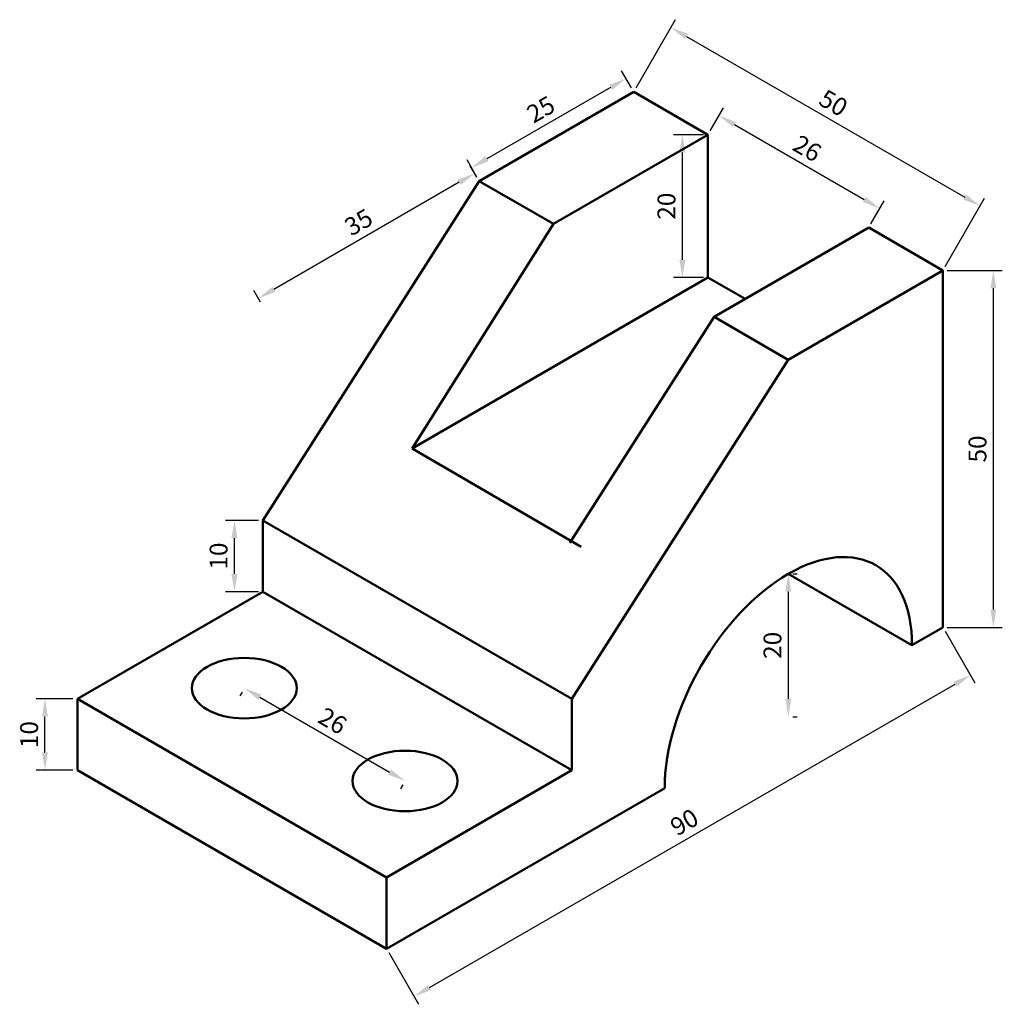
# Model space of a CAD drawing. Units: millimetres. Extents: x 2685 to 2823, y 469 to 607.
import ezdxf

# ---------------------------------------------------------------- set-up
doc = ezdxf.new("R2010")
doc.units = ezdxf.units.MM
doc.layers.add('M-DIMS', color=2, linetype='Continuous', lineweight=25)
doc.layers.add('M-OUTL', color=7, linetype='Continuous', lineweight=50)
doc.styles.get("Standard").update_dxf_attribs({"font": 'arial.ttf'})
doc.dimstyles.new('ISO-25', dxfattribs={"dimtxt": 2.5, "dimasz": 2.5, "dimexe": 1.25, "dimexo": 0.625, "dimtad": 1, "dimtxsty": 'Standard', "dimcen": 2.5, "dimadec": 0, "dimazin": 0, "dimtfac": 1, "dimtmove": 0, "dimatfit": 3, "dimfxl": 1, "dimarcsym": 0})

# ---------------------------------------------------------------- blocks, each defined once
blk = doc.blocks.new('*D1')
at = {"layer": 'Defpoints', "color": 0, "transparency": 16777216}
for p in [(2792.76, 529.56), (2792.76, 529.56), (2792.76, 509.56)]:
    blk.add_point(p, dxfattribs=at)
at = {"layer": 'M-DIMS', "color": 0, "lineweight": -2, "transparency": 16777216}
for p, q in [((2793.38, 529.56), (2794.01, 529.56)), ((2792.76, 512.06), (2792.76, 527.06)), ((2793.38, 509.56), (2794.01, 509.56))]:
    blk.add_line(p, q, dxfattribs=at)
at = {"layer": 'M-DIMS', "color": 0, "transparency": 16777216}
for points in [[(2792.34, 527.06), (2793.17, 527.06), (2792.76, 529.56)], [(2792.34, 512.06), (2793.17, 512.06), (2792.76, 509.56)]]:
    blk.add_solid(points, dxfattribs=at)
at = {"layer": 'M-DIMS', "color": 0, "transparency": 16777216, "insert": (2790.86, 519.56), "char_height": 2.5, "attachment_point": 5, "rotation": 90}
blk.add_mtext('20', dxfattribs=at)
blk = doc.blocks.new('*D2')
at = {"layer": 'Defpoints', "color": 0, "transparency": 16777216}
for p in [(2814.41, 572.06), (2821.48, 572.06), (2814.41, 522.06)]:
    blk.add_point(p, dxfattribs=at)
at = {"layer": 'M-DIMS', "color": 0, "lineweight": -2, "transparency": 16777216}
for p, q in [((2815.03, 572.06), (2822.73, 572.06)), ((2821.48, 524.56), (2821.48, 569.56)), ((2815.03, 522.06), (2822.73, 522.06))]:
    blk.add_line(p, q, dxfattribs=at)
at = {"layer": 'M-DIMS', "color": 0, "transparency": 16777216}
for points in [[(2821.07, 569.56), (2821.9, 569.56), (2821.48, 572.06)], [(2821.07, 524.56), (2821.9, 524.56), (2821.48, 522.06)]]:
    blk.add_solid(points, dxfattribs=at)
at = {"layer": 'M-DIMS', "color": 0, "transparency": 16777216, "insert": (2819.58, 547.06), "char_height": 2.5, "attachment_point": 5, "rotation": 90}
blk.add_mtext('50', dxfattribs=at)
blk = doc.blocks.new('*D3')
at = {"layer": 'Defpoints', "color": 0, "transparency": 16777216}
for p in [(2781.5, 591.06), (2777.91, 571.06), (2781.5, 571.06)]:
    blk.add_point(p, dxfattribs=at)
at = {"layer": 'M-DIMS', "color": 0, "lineweight": -2, "transparency": 16777216}
for p, q in [((2780.87, 591.06), (2776.66, 591.06)), ((2777.91, 588.56), (2777.91, 573.56)), ((2780.87, 571.06), (2776.66, 571.06))]:
    blk.add_line(p, q, dxfattribs=at)
at = {"layer": 'M-DIMS', "color": 0, "transparency": 16777216}
for points in [[(2777.5, 588.56), (2778.33, 588.56), (2777.91, 591.06)], [(2777.5, 573.56), (2778.33, 573.56), (2777.91, 571.06)]]:
    blk.add_solid(points, dxfattribs=at)
at = {"layer": 'M-DIMS', "color": 0, "transparency": 16777216, "insert": (2776.01, 581.06), "char_height": 2.5, "attachment_point": 5, "rotation": 90}
blk.add_mtext('20', dxfattribs=at)
blk = doc.blocks.new('*D4')
at = {"layer": 'Defpoints', "color": 0, "transparency": 16777216}
for p in [(2749.46, 584.56), (2718.52, 568.15), (2719.15, 567.06)]:
    blk.add_point(p, dxfattribs=at)
at = {"layer": 'M-DIMS', "color": 0, "lineweight": -2, "transparency": 16777216}
for p, q in [((2749.14, 585.11), (2748.21, 586.73)), ((2746.67, 584.4), (2720.69, 569.4)), ((2718.83, 567.61), (2717.9, 569.23))]:
    blk.add_line(p, q, dxfattribs=at)
at = {"layer": 'M-DIMS', "color": 0, "transparency": 16777216}
for points in [[(2746.46, 584.76), (2746.87, 584.04), (2748.83, 585.65)], [(2720.48, 569.76), (2720.89, 569.04), (2718.52, 568.15)]]:
    blk.add_solid(points, dxfattribs=at)
at = {"layer": 'M-DIMS', "color": 0, "transparency": 16777216, "insert": (2732.72, 578.54), "char_height": 2.5, "attachment_point": 5, "rotation": 30}
blk.add_mtext('35', dxfattribs=at)
blk = doc.blocks.new('*D5')
at = {"layer": 'Defpoints', "color": 0, "transparency": 16777216}
for p in [(2771.11, 597.06), (2748.37, 586.44), (2749.46, 584.56)]:
    blk.add_point(p, dxfattribs=at)
at = {"layer": 'M-DIMS', "color": 0, "lineweight": -2, "transparency": 16777216}
for p, q in [((2770.79, 597.61), (2769.4, 600.03)), ((2767.86, 597.69), (2750.54, 587.69)), ((2749.14, 585.11), (2747.75, 587.53))]:
    blk.add_line(p, q, dxfattribs=at)
at = {"layer": 'M-DIMS', "color": 0, "transparency": 16777216}
for points in [[(2767.65, 598.05), (2768.07, 597.33), (2770.02, 598.94)], [(2750.33, 588.05), (2750.75, 587.33), (2748.37, 586.44)]]:
    blk.add_solid(points, dxfattribs=at)
at = {"layer": 'M-DIMS', "color": 0, "transparency": 16777216, "insert": (2758.25, 594.34), "char_height": 2.5, "attachment_point": 5, "rotation": 30}
blk.add_mtext('25', dxfattribs=at)
blk = doc.blocks.new('*D6')
at = {"layer": 'Defpoints', "color": 0, "transparency": 16777216}
for p in [(2781.5, 591.06), (2805.56, 580.74), (2804.02, 578.06)]:
    blk.add_point(p, dxfattribs=at)
at = {"layer": 'M-DIMS', "color": 0, "lineweight": -2, "transparency": 16777216}
for p, q in [((2781.81, 591.61), (2783.67, 594.82)), ((2785.21, 592.49), (2803.39, 581.99)), ((2804.33, 578.61), (2806.18, 581.82))]:
    blk.add_line(p, q, dxfattribs=at)
at = {"layer": 'M-DIMS', "color": 0, "transparency": 16777216}
for points in [[(2785.42, 592.85), (2785, 592.13), (2783.04, 593.74)], [(2803.6, 582.35), (2803.19, 581.63), (2805.56, 580.74)]]:
    blk.add_solid(points, dxfattribs=at)
at = {"layer": 'M-DIMS', "color": 0, "transparency": 16777216, "insert": (2795.25, 588.88), "char_height": 2.5, "attachment_point": 5, "rotation": 330}
blk.add_mtext('26', dxfattribs=at)
blk = doc.blocks.new('*D7')
at = {"layer": 'Defpoints', "color": 0, "transparency": 16777216}
for p in [(2771.11, 597.06), (2819.62, 581.09), (2814.41, 572.06)]:
    blk.add_point(p, dxfattribs=at)
at = {"layer": 'M-DIMS', "color": 0, "lineweight": -2, "transparency": 16777216}
for p, q in [((2771.42, 597.61), (2776.94, 607.18)), ((2778.48, 604.84), (2817.46, 582.34)), ((2814.72, 572.61), (2820.25, 582.18))]:
    blk.add_line(p, q, dxfattribs=at)
at = {"layer": 'M-DIMS', "color": 0, "transparency": 16777216}
for points in [[(2778.69, 605.2), (2778.28, 604.48), (2776.32, 606.09)], [(2817.66, 582.7), (2817.25, 581.98), (2819.62, 581.09)]]:
    blk.add_solid(points, dxfattribs=at)
at = {"layer": 'M-DIMS', "color": 0, "transparency": 16777216, "insert": (2798.92, 595.24), "char_height": 2.5, "attachment_point": 5, "rotation": 330}
blk.add_mtext('50', dxfattribs=at)
blk = doc.blocks.new('*D8')
at = {"layer": 'Defpoints', "color": 0, "transparency": 16777216}
for p in [(2814.41, 522.06), (2818.27, 515.37), (2736.47, 477.06)]:
    blk.add_point(p, dxfattribs=at)
at = {"layer": 'M-DIMS', "color": 0, "lineweight": -2, "transparency": 16777216}
for p, q in [((2814.72, 521.52), (2818.9, 514.29)), ((2742.5, 471.62), (2816.11, 514.12)), ((2736.78, 476.52), (2740.96, 469.29))]:
    blk.add_line(p, q, dxfattribs=at)
at = {"layer": 'M-DIMS', "color": 0, "transparency": 16777216}
for points in [[(2815.9, 514.48), (2816.32, 513.76), (2818.27, 515.37)], [(2742.29, 471.98), (2742.7, 471.26), (2740.33, 470.37)]]:
    blk.add_solid(points, dxfattribs=at)
at = {"layer": 'M-DIMS', "color": 0, "transparency": 16777216, "insert": (2778.35, 494.52), "char_height": 2.5, "attachment_point": 5, "rotation": 30}
blk.add_mtext('90', dxfattribs=at)
blk = doc.blocks.new('*D9')
at = {"layer": 'Defpoints', "color": 0, "transparency": 16777216}
for p in [(2688.63, 512.06), (2693.16, 512.06), (2693.16, 502.06)]:
    blk.add_point(p, dxfattribs=at)
at = {"layer": 'M-DIMS', "color": 0, "lineweight": -2, "transparency": 16777216}
for p, q in [((2692.54, 512.06), (2687.38, 512.06)), ((2688.63, 504.56), (2688.63, 509.56)), ((2692.54, 502.06), (2687.38, 502.06))]:
    blk.add_line(p, q, dxfattribs=at)
at = {"layer": 'M-DIMS', "color": 0, "transparency": 16777216}
for points in [[(2688.21, 509.56), (2689.04, 509.56), (2688.63, 512.06)], [(2688.21, 504.56), (2689.04, 504.56), (2688.63, 502.06)]]:
    blk.add_solid(points, dxfattribs=at)
at = {"layer": 'M-DIMS', "color": 0, "transparency": 16777216, "insert": (2686.73, 507.06), "char_height": 2.5, "attachment_point": 5, "rotation": 90}
blk.add_mtext('10', dxfattribs=at)
blk = doc.blocks.new('*D10')
at = {"layer": 'Defpoints', "color": 0, "transparency": 16777216}
for p in [(2715.17, 537.06), (2719.15, 537.06), (2719.15, 527.06)]:
    blk.add_point(p, dxfattribs=at)
at = {"layer": 'M-DIMS', "color": 0, "lineweight": -2, "transparency": 16777216}
for p, q in [((2718.52, 537.06), (2713.92, 537.06)), ((2715.17, 529.56), (2715.17, 534.56)), ((2718.52, 527.06), (2713.92, 527.06))]:
    blk.add_line(p, q, dxfattribs=at)
at = {"layer": 'M-DIMS', "color": 0, "transparency": 16777216}
for points in [[(2714.75, 534.56), (2715.59, 534.56), (2715.17, 537.06)], [(2714.75, 529.56), (2715.59, 529.56), (2715.17, 527.06)]]:
    blk.add_solid(points, dxfattribs=at)
at = {"layer": 'M-DIMS', "color": 0, "transparency": 16777216, "insert": (2713.27, 532.06), "char_height": 2.5, "attachment_point": 5, "rotation": 90}
blk.add_mtext('10', dxfattribs=at)
blk = doc.blocks.new('*D11')
at = {"layer": 'Defpoints', "color": 0, "transparency": 16777216}
for p in [(2716.55, 513.56), (2739.06, 500.56), (2739.06, 500.56)]:
    blk.add_point(p, dxfattribs=at)
at = {"layer": 'M-DIMS', "color": 0, "lineweight": -2, "transparency": 16777216}
for p, q in [((2716.23, 513.02), (2715.92, 512.48)), ((2718.71, 512.31), (2736.9, 501.81)), ((2738.75, 500.02), (2738.44, 499.48))]:
    blk.add_line(p, q, dxfattribs=at)
at = {"layer": 'M-DIMS', "color": 0, "transparency": 16777216}
for points in [[(2718.92, 512.68), (2718.5, 511.95), (2716.55, 513.56)], [(2737.11, 502.18), (2736.69, 501.45), (2739.06, 500.56)]]:
    blk.add_solid(points, dxfattribs=at)
at = {"layer": 'M-DIMS', "color": 0, "transparency": 16777216, "insert": (2728.76, 508.71), "char_height": 2.5, "attachment_point": 5, "rotation": 330}
blk.add_mtext('26', dxfattribs=at)

msp = doc.modelspace()

# ---------------------------------------------------------------- linework, layer by layer
at = {"layer": 'M-OUTL'}
for p, q in [((2771.107, 597.064), (2749.456, 584.564)), ((2781.499, 591.064), (2771.107, 597.064)), ((2759.849, 578.564), (2781.499, 591.064)), ((2781.499, 591.064), (2781.499, 571.064)), ((2749.456, 584.564), (2719.145, 537.064)), ((2749.456, 584.564), (2759.849, 578.564)), ((2759.849, 578.564), (2740.043, 547.13)), ((2782.365, 565.564), (2804.016, 578.064)), ((2804.016, 578.064), (2814.408, 572.064)), ((2781.499, 571.064), (2740.043, 547.13)), ((2781.499, 571.064), (2786.695, 568.064)), ((2814.408, 572.064), (2792.758, 559.564)), ((2814.408, 522.064), (2814.408, 572.064)), ((2782.365, 565.564), (2762.158, 533.898)), ((2792.758, 559.564), (2782.365, 565.564)), ((2762.447, 512.064), (2792.758, 559.564)), ((2740.043, 547.13), (2763.761, 533.34)), ((2762.447, 512.064), (2719.145, 537.064)), ((2719.145, 537.064), (2719.145, 527.064)), ((2810.078, 519.564), (2792.758, 529.564)), ((2719.145, 527.064), (2693.165, 512.064)), ((2719.145, 527.064), (2762.447, 502.064)), ((2814.408, 522.064), (2810.078, 519.564)), ((2810.078, 519.564), (2814.408, 522.064)), ((2736.466, 487.064), (2693.165, 512.064)), ((2693.165, 512.064), (2693.165, 502.064)), ((2762.447, 502.064), (2762.447, 512.064)), ((2693.165, 502.064), (2736.466, 477.064)), ((2736.466, 487.064), (2762.447, 502.064)), ((2736.466, 477.064), (2775.437, 499.564)), ((2736.466, 477.064), (2736.466, 487.064))]:
    msp.add_line(p, q, dxfattribs=at)
msp.add_ellipse((2792.758, 509.564), major_axis=(-12.247, -21.213), ratio=0.5773503, start_param=2.3561945, end_param=5.4977871, dxfattribs=at)
for centre in [(2716.547, 513.564), (2739.064, 500.564)]:
    msp.add_ellipse(centre, major_axis=(-7.348, 0), ratio=0.5773503, dxfattribs=at)

# ---------------------------------------------------------------- dimensions: what is measured, and where the dimension line sits
at = {"layer": 'M-DIMS'}
for p1, p2, distance, picture, middle in [((2771.107, 597.064), (2814.408, 572.064), 10.426, '*D7', (2798.921, 595.24)), ((2771.107, 597.064), (2749.456, 584.564), -2.169, '*D5', (2758.246, 594.34)), ((2781.499, 591.064), (2804.016, 578.064), 3.087, '*D6', (2795.252, 588.884)), ((2749.456, 584.564), (2719.145, 567.064), -1.25, '*D4', (2732.725, 578.544)), ((2736.466, 477.064), (2814.408, 522.064), -7.73, '*D8', (2778.351, 494.517)), ((2716.547, 513.564), (2739.064, 500.564), 0, '*D11', (2728.756, 508.711))]:
    dim = msp.add_aligned_dim(p1=p1, p2=p2, distance=distance, dimstyle='ISO-25', override={"dimclrd": 0, "dimclre": 0, "dimclrt": 0}, dxfattribs=at)
    dim.commit()
    dim.dimension.update_dxf_attribs({"geometry": picture, "text_midpoint": middle})
for base, p1, p2, picture, middle in [((2777.914, 571.064), (2781.499, 591.064), (2781.499, 571.064), '*D3', (2776.012, 581.064)), ((2821.483, 572.064), (2814.408, 522.064), (2814.408, 572.064), '*D2', (2819.581, 547.064)), ((2715.168, 537.064), (2719.145, 527.064), (2719.145, 537.064), '*D10', (2713.267, 532.064)), ((2792.758, 529.564), (2792.758, 509.564), (2792.758, 529.564), '*D1', (2790.856, 519.564)), ((2688.628, 512.064), (2693.165, 502.064), (2693.165, 512.064), '*D9', (2686.727, 507.064))]:
    dim = msp.add_linear_dim(base=base, p1=p1, p2=p2, angle=90, dimstyle='ISO-25', override={"dimclrd": 0, "dimclre": 0, "dimclrt": 0}, dxfattribs=at)
    dim.commit()
    dim.dimension.update_dxf_attribs({"geometry": picture, "text_midpoint": middle})

doc.saveas('drawing.dxf')
